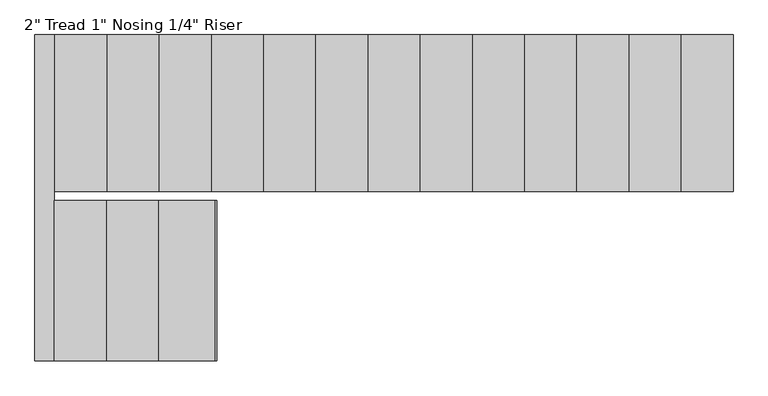
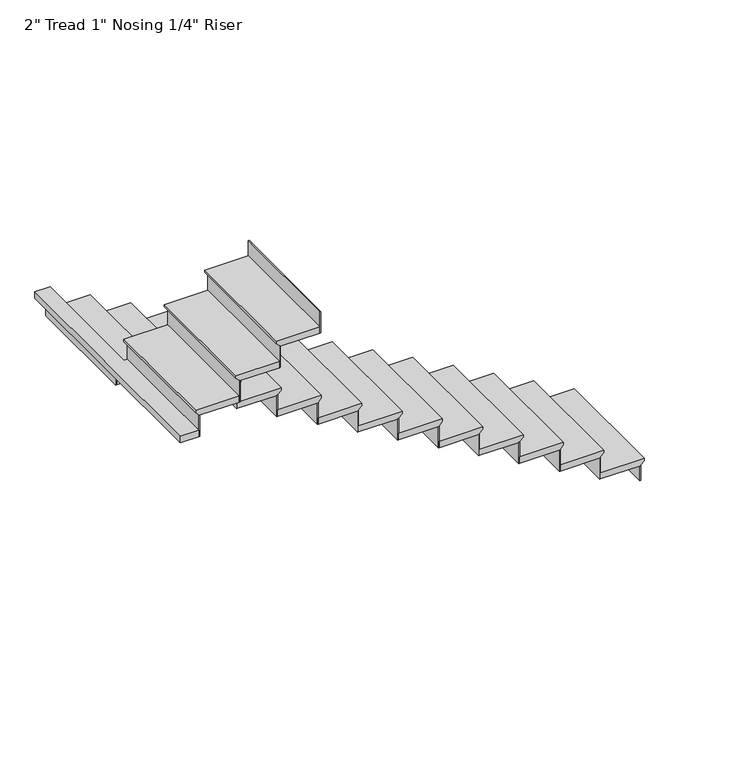
"""IFC4 building model written with IfcOpenShell, lengths in millimetres: stair flight geometry."""

from ifc_helpers import new_model, si_unit, origin, place, context, project, spatial, faceted_brep, source, transform, mapped, element, save


def stair_flight_91c59d30(model_context):
    return source(origin(), model_context, "Body", "Brep", [
        faceted_brep([(6794.5, 11386.0372886, 150.2833333), (6794.5, 11386.0372886, 169.3333333), (6794.5, 10471.6372886, 169.3333333), (6794.5, 10471.6372886, 150.2833333), (6769.1, 11386.0372886, 124.8833333), (6769.1, 10471.6372886, 124.8833333), (6464.3, 11386.0372886, 169.3333333), (6464.3, 10471.6372886, 169.3333333), (6769.1, 10471.6372886, 118.5333333), (6464.3, 10471.6372886, 118.5333333), (6464.3, 11386.0372886, 118.5333333), (6769.1, 11386.0372886, 118.5333333)], [[[0, 1, 2, 3]], [[4, 0, 3, 5]], [[2, 1, 6, 7]], [[8, 9, 10, 11]], [[2, 7, 9, 8, 5, 3]], [[8, 11, 4, 5]], [[6, 1, 0, 4, 11, 10]], [[7, 6, 10, 9]]]),
        faceted_brep([(6769.1, 11386.0372886, 118.5333333), (6769.1, 11386.0372886, 0.0), (6762.75, 11386.0372886, 0.0), (6762.75, 11386.0372886, 118.5333333), (6769.1, 10471.6372886, 118.5333333), (6762.75, 10471.6372886, 118.5333333), (6762.75, 10471.6372886, 0.0), (6769.1, 10471.6372886, 0.0)], [[[0, 1, 2, 3]], [[4, 5, 6, 7]], [[1, 0, 4, 7]], [[2, 1, 7, 6]], [[3, 2, 6, 5]], [[0, 3, 5, 4]]]),
        faceted_brep([(6464.3, 11386.0372886, 287.8666667), (6464.3, 11386.0372886, 118.5333333), (6457.95, 11386.0372886, 118.5333333), (6457.95, 11386.0372886, 287.8666667), (6464.3, 10471.6372886, 287.8666667), (6457.95, 10471.6372886, 287.8666667), (6457.95, 10471.6372886, 118.5333333), (6464.3, 10471.6372886, 118.5333333)], [[[0, 1, 2, 3]], [[4, 5, 6, 7]], [[1, 0, 4, 7]], [[2, 1, 7, 6]], [[3, 2, 6, 5]], [[0, 3, 5, 4]]]),
        faceted_brep([(6489.7, 10471.6372886, 338.6666667), (6489.7, 11386.0372886, 338.6666667), (6159.5, 11386.0372886, 338.6666667), (6159.5, 10471.6372886, 338.6666667), (6464.3, 10471.6372886, 287.8666667), (6159.5, 10471.6372886, 287.8666667), (6159.5, 11386.0372886, 287.8666667), (6464.3, 11386.0372886, 287.8666667), (6464.3, 10471.6372886, 294.2166667), (6489.7, 10471.6372886, 319.6166667), (6464.3, 11386.0372886, 294.2166667), (6489.7, 11386.0372886, 319.6166667)], [[[0, 1, 2, 3]], [[4, 5, 6, 7]], [[0, 3, 5, 4, 8, 9]], [[4, 7, 10, 8]], [[2, 1, 11, 10, 7, 6]], [[3, 2, 6, 5]], [[11, 1, 0, 9]], [[10, 11, 9, 8]]]),
        faceted_brep([(6159.5, 11386.0372886, 457.2), (6159.5, 11386.0372886, 287.8666667), (6153.15, 11386.0372886, 287.8666667), (6153.15, 11386.0372886, 457.2), (6159.5, 10471.6372886, 457.2), (6153.15, 10471.6372886, 457.2), (6153.15, 10471.6372886, 287.8666667), (6159.5, 10471.6372886, 287.8666667)], [[[0, 1, 2, 3]], [[4, 5, 6, 7]], [[1, 0, 4, 7]], [[2, 1, 7, 6]], [[3, 2, 6, 5]], [[0, 3, 5, 4]]]),
        faceted_brep([(6184.9, 10471.6372886, 508.0), (6184.9, 11386.0372886, 508.0), (5854.7, 11386.0372886, 508.0), (5854.7, 10471.6372886, 508.0), (6159.5, 10471.6372886, 457.2), (5854.7, 10471.6372886, 457.2), (5854.7, 11386.0372886, 457.2), (6159.5, 11386.0372886, 457.2), (6159.5, 10471.6372886, 463.55), (6184.9, 10471.6372886, 488.95), (6159.5, 11386.0372886, 463.55), (6184.9, 11386.0372886, 488.95)], [[[0, 1, 2, 3]], [[4, 5, 6, 7]], [[0, 3, 5, 4, 8, 9]], [[4, 7, 10, 8]], [[2, 1, 11, 10, 7, 6]], [[3, 2, 6, 5]], [[11, 1, 0, 9]], [[10, 11, 9, 8]]]),
        faceted_brep([(5854.7, 11386.0372886, 626.5333333), (5854.7, 11386.0372886, 457.2), (5848.35, 11386.0372886, 457.2), (5848.35, 11386.0372886, 626.5333333), (5854.7, 10471.6372886, 626.5333333), (5848.35, 10471.6372886, 626.5333333), (5848.35, 10471.6372886, 457.2), (5854.7, 10471.6372886, 457.2)], [[[0, 1, 2, 3]], [[4, 5, 6, 7]], [[1, 0, 4, 7]], [[2, 1, 7, 6]], [[3, 2, 6, 5]], [[0, 3, 5, 4]]]),
        faceted_brep([(5880.1, 10471.6372886, 677.3333333), (5880.1, 11386.0372886, 677.3333333), (5549.9, 11386.0372886, 677.3333333), (5549.9, 10471.6372886, 677.3333333), (5854.7, 10471.6372886, 626.5333333), (5549.9, 10471.6372886, 626.5333333), (5549.9, 11386.0372886, 626.5333333), (5854.7, 11386.0372886, 626.5333333), (5854.7, 10471.6372886, 632.8833333), (5880.1, 10471.6372886, 658.2833333), (5854.7, 11386.0372886, 632.8833333), (5880.1, 11386.0372886, 658.2833333)], [[[0, 1, 2, 3]], [[4, 5, 6, 7]], [[0, 3, 5, 4, 8, 9]], [[4, 7, 10, 8]], [[2, 1, 11, 10, 7, 6]], [[3, 2, 6, 5]], [[11, 1, 0, 9]], [[10, 11, 9, 8]]]),
        faceted_brep([(5549.9, 11386.0372886, 795.8666667), (5549.9, 11386.0372886, 626.5333333), (5543.55, 11386.0372886, 626.5333333), (5543.55, 11386.0372886, 795.8666667), (5549.9, 10471.6372886, 795.8666667), (5543.55, 10471.6372886, 795.8666667), (5543.55, 10471.6372886, 626.5333333), (5549.9, 10471.6372886, 626.5333333)], [[[0, 1, 2, 3]], [[4, 5, 6, 7]], [[1, 0, 4, 7]], [[2, 1, 7, 6]], [[3, 2, 6, 5]], [[0, 3, 5, 4]]]),
        faceted_brep([(5575.3, 10471.6372886, 846.6666667), (5575.3, 11386.0372886, 846.6666667), (5245.1, 11386.0372886, 846.6666667), (5245.1, 10471.6372886, 846.6666667), (5549.9, 10471.6372886, 795.8666667), (5245.1, 10471.6372886, 795.8666667), (5245.1, 11386.0372886, 795.8666667), (5549.9, 11386.0372886, 795.8666667), (5549.9, 10471.6372886, 802.2166667), (5575.3, 10471.6372886, 827.6166667), (5549.9, 11386.0372886, 802.2166667), (5575.3, 11386.0372886, 827.6166667)], [[[0, 1, 2, 3]], [[4, 5, 6, 7]], [[0, 3, 5, 4, 8, 9]], [[4, 7, 10, 8]], [[2, 1, 11, 10, 7, 6]], [[3, 2, 6, 5]], [[11, 1, 0, 9]], [[10, 11, 9, 8]]]),
        faceted_brep([(5245.1, 11386.0372886, 965.2), (5245.1, 11386.0372886, 795.8666667), (5238.75, 11386.0372886, 795.8666667), (5238.75, 11386.0372886, 965.2), (5245.1, 10471.6372886, 965.2), (5238.75, 10471.6372886, 965.2), (5238.75, 10471.6372886, 795.8666667), (5245.1, 10471.6372886, 795.8666667)], [[[0, 1, 2, 3]], [[4, 5, 6, 7]], [[1, 0, 4, 7]], [[2, 1, 7, 6]], [[3, 2, 6, 5]], [[0, 3, 5, 4]]]),
        faceted_brep([(5270.5, 10471.6372886, 1016.0), (5270.5, 11386.0372886, 1016.0), (4940.3, 11386.0372886, 1016.0), (4940.3, 10471.6372886, 1016.0), (5245.1, 10471.6372886, 965.2), (4940.3, 10471.6372886, 965.2), (4940.3, 11386.0372886, 965.2), (5245.1, 11386.0372886, 965.2), (5245.1, 10471.6372886, 971.55), (5270.5, 10471.6372886, 996.95), (5245.1, 11386.0372886, 971.55), (5270.5, 11386.0372886, 996.95)], [[[0, 1, 2, 3]], [[4, 5, 6, 7]], [[0, 3, 5, 4, 8, 9]], [[4, 7, 10, 8]], [[2, 1, 11, 10, 7, 6]], [[3, 2, 6, 5]], [[11, 1, 0, 9]], [[10, 11, 9, 8]]]),
        faceted_brep([(4940.3, 11386.0372886, 1134.5333333), (4940.3, 11386.0372886, 965.2), (4933.95, 11386.0372886, 965.2), (4933.95, 11386.0372886, 1134.5333333), (4940.3, 10471.6372886, 1134.5333333), (4933.95, 10471.6372886, 1134.5333333), (4933.95, 10471.6372886, 965.2), (4940.3, 10471.6372886, 965.2)], [[[0, 1, 2, 3]], [[4, 5, 6, 7]], [[1, 0, 4, 7]], [[2, 1, 7, 6]], [[3, 2, 6, 5]], [[0, 3, 5, 4]]]),
        faceted_brep([(4965.7, 10471.6372886, 1185.3333333), (4965.7, 11386.0372886, 1185.3333333), (4635.5, 11386.0372886, 1185.3333333), (4635.5, 10471.6372886, 1185.3333333), (4940.3, 10471.6372886, 1134.5333333), (4635.5, 10471.6372886, 1134.5333333), (4635.5, 11386.0372886, 1134.5333333), (4940.3, 11386.0372886, 1134.5333333), (4940.3, 10471.6372886, 1140.8833333), (4965.7, 10471.6372886, 1166.2833333), (4940.3, 11386.0372886, 1140.8833333), (4965.7, 11386.0372886, 1166.2833333)], [[[0, 1, 2, 3]], [[4, 5, 6, 7]], [[0, 3, 5, 4, 8, 9]], [[4, 7, 10, 8]], [[2, 1, 11, 10, 7, 6]], [[3, 2, 6, 5]], [[11, 1, 0, 9]], [[10, 11, 9, 8]]]),
        faceted_brep([(4635.5, 11386.0372886, 1303.8666667), (4635.5, 11386.0372886, 1134.5333333), (4629.15, 11386.0372886, 1134.5333333), (4629.15, 11386.0372886, 1303.8666667), (4635.5, 10471.6372886, 1303.8666667), (4629.15, 10471.6372886, 1303.8666667), (4629.15, 10471.6372886, 1134.5333333), (4635.5, 10471.6372886, 1134.5333333)], [[[0, 1, 2, 3]], [[4, 5, 6, 7]], [[1, 0, 4, 7]], [[2, 1, 7, 6]], [[3, 2, 6, 5]], [[0, 3, 5, 4]]]),
        faceted_brep([(4660.9, 10471.6372886, 1354.6666667), (4660.9, 11386.0372886, 1354.6666667), (4330.7, 11386.0372886, 1354.6666667), (4330.7, 10471.6372886, 1354.6666667), (4635.5, 10471.6372886, 1303.8666667), (4330.7, 10471.6372886, 1303.8666667), (4330.7, 11386.0372886, 1303.8666667), (4635.5, 11386.0372886, 1303.8666667), (4635.5, 10471.6372886, 1310.2166667), (4660.9, 10471.6372886, 1335.6166667), (4635.5, 11386.0372886, 1310.2166667), (4660.9, 11386.0372886, 1335.6166667)], [[[0, 1, 2, 3]], [[4, 5, 6, 7]], [[0, 3, 5, 4, 8, 9]], [[4, 7, 10, 8]], [[2, 1, 11, 10, 7, 6]], [[3, 2, 6, 5]], [[11, 1, 0, 9]], [[10, 11, 9, 8]]]),
        faceted_brep([(4330.7, 11386.0372886, 1473.2), (4330.7, 11386.0372886, 1303.8666667), (4324.35, 11386.0372886, 1303.8666667), (4324.35, 11386.0372886, 1473.2), (4330.7, 10471.6372886, 1473.2), (4324.35, 10471.6372886, 1473.2), (4324.35, 10471.6372886, 1303.8666667), (4330.7, 10471.6372886, 1303.8666667)], [[[0, 1, 2, 3]], [[4, 5, 6, 7]], [[1, 0, 4, 7]], [[2, 1, 7, 6]], [[3, 2, 6, 5]], [[0, 3, 5, 4]]]),
        faceted_brep([(4356.1, 10471.6372886, 1524.0), (4356.1, 11386.0372886, 1524.0), (4025.9, 11386.0372886, 1524.0), (4025.9, 10471.6372886, 1524.0), (4330.7, 10471.6372886, 1473.2), (4025.9, 10471.6372886, 1473.2), (4025.9, 11386.0372886, 1473.2), (4330.7, 11386.0372886, 1473.2), (4330.7, 10471.6372886, 1479.55), (4356.1, 10471.6372886, 1504.95), (4330.7, 11386.0372886, 1479.55), (4356.1, 11386.0372886, 1504.95)], [[[0, 1, 2, 3]], [[4, 5, 6, 7]], [[0, 3, 5, 4, 8, 9]], [[4, 7, 10, 8]], [[2, 1, 11, 10, 7, 6]], [[3, 2, 6, 5]], [[11, 1, 0, 9]], [[10, 11, 9, 8]]]),
        faceted_brep([(4025.9, 11386.0372886, 1642.5333333), (4025.9, 11386.0372886, 1473.2), (4019.55, 11386.0372886, 1473.2), (4019.55, 11386.0372886, 1642.5333333), (4025.9, 10471.6372886, 1642.5333333), (4019.55, 10471.6372886, 1642.5333333), (4019.55, 10471.6372886, 1473.2), (4025.9, 10471.6372886, 1473.2)], [[[0, 1, 2, 3]], [[4, 5, 6, 7]], [[1, 0, 4, 7]], [[2, 1, 7, 6]], [[3, 2, 6, 5]], [[0, 3, 5, 4]]]),
        faceted_brep([(4051.3, 10471.6372886, 1693.3333333), (4051.3, 11386.0372886, 1693.3333333), (3721.1, 11386.0372886, 1693.3333333), (3721.1, 10471.6372886, 1693.3333333), (4025.9, 10471.6372886, 1642.5333333), (3721.1, 10471.6372886, 1642.5333333), (3721.1, 11386.0372886, 1642.5333333), (4025.9, 11386.0372886, 1642.5333333), (4025.9, 10471.6372886, 1648.8833333), (4051.3, 10471.6372886, 1674.2833333), (4025.9, 11386.0372886, 1648.8833333), (4051.3, 11386.0372886, 1674.2833333)], [[[0, 1, 2, 3]], [[4, 5, 6, 7]], [[0, 3, 5, 4, 8, 9]], [[4, 7, 10, 8]], [[2, 1, 11, 10, 7, 6]], [[3, 2, 6, 5]], [[11, 1, 0, 9]], [[10, 11, 9, 8]]]),
        faceted_brep([(3721.1, 11386.0372886, 1811.8666667), (3721.1, 11386.0372886, 1642.5333333), (3714.75, 11386.0372886, 1642.5333333), (3714.75, 11386.0372886, 1811.8666667), (3721.1, 10471.6372886, 1811.8666667), (3714.75, 10471.6372886, 1811.8666667), (3714.75, 10471.6372886, 1642.5333333), (3721.1, 10471.6372886, 1642.5333333)], [[[0, 1, 2, 3]], [[4, 5, 6, 7]], [[1, 0, 4, 7]], [[2, 1, 7, 6]], [[3, 2, 6, 5]], [[0, 3, 5, 4]]]),
        faceted_brep([(3746.5, 10471.6372886, 1862.6666667), (3746.5, 11386.0372886, 1862.6666667), (3416.3, 11386.0372886, 1862.6666667), (3416.3, 10471.6372886, 1862.6666667), (3721.1, 10471.6372886, 1811.8666667), (3416.3, 10471.6372886, 1811.8666667), (3416.3, 11386.0372886, 1811.8666667), (3721.1, 11386.0372886, 1811.8666667), (3721.1, 10471.6372886, 1818.2166667), (3746.5, 10471.6372886, 1843.6166667), (3721.1, 11386.0372886, 1818.2166667), (3746.5, 11386.0372886, 1843.6166667)], [[[0, 1, 2, 3]], [[4, 5, 6, 7]], [[0, 3, 5, 4, 8, 9]], [[4, 7, 10, 8]], [[2, 1, 11, 10, 7, 6]], [[3, 2, 6, 5]], [[11, 1, 0, 9]], [[10, 11, 9, 8]]]),
        faceted_brep([(3416.3, 11386.0372886, 1981.2), (3416.3, 11386.0372886, 1811.8666667), (3409.95, 11386.0372886, 1811.8666667), (3409.95, 11386.0372886, 1981.2), (3416.3, 10471.6372886, 1981.2), (3409.95, 10471.6372886, 1981.2), (3409.95, 10471.6372886, 1811.8666667), (3416.3, 10471.6372886, 1811.8666667)], [[[0, 1, 2, 3]], [[4, 5, 6, 7]], [[1, 0, 4, 7]], [[2, 1, 7, 6]], [[3, 2, 6, 5]], [[0, 3, 5, 4]]]),
        faceted_brep([(3441.7, 10471.6372886, 2032.0), (3441.7, 11386.0372886, 2032.0), (3111.5, 11386.0372886, 2032.0), (3111.5, 10471.6372886, 2032.0), (3416.3, 10471.6372886, 1981.2), (3111.5, 10471.6372886, 1981.2), (3111.5, 11386.0372886, 1981.2), (3416.3, 11386.0372886, 1981.2), (3416.3, 10471.6372886, 1987.55), (3441.7, 10471.6372886, 2012.95), (3416.3, 11386.0372886, 1987.55), (3441.7, 11386.0372886, 2012.95)], [[[0, 1, 2, 3]], [[4, 5, 6, 7]], [[0, 3, 5, 4, 8, 9]], [[4, 7, 10, 8]], [[2, 1, 11, 10, 7, 6]], [[3, 2, 6, 5]], [[11, 1, 0, 9]], [[10, 11, 9, 8]]]),
        faceted_brep([(3111.5, 11386.0372886, 2150.5333333), (3111.5, 11386.0372886, 1981.2), (3105.15, 11386.0372886, 1981.2), (3105.15, 11386.0372886, 2150.5333333), (3111.5, 10471.6372886, 2150.5333333), (3105.15, 10471.6372886, 2150.5333333), (3105.15, 10471.6372886, 1981.2), (3111.5, 10471.6372886, 1981.2)], [[[0, 1, 2, 3]], [[4, 5, 6, 7]], [[1, 0, 4, 7]], [[2, 1, 7, 6]], [[3, 2, 6, 5]], [[0, 3, 5, 4]]]),
        faceted_brep([(3136.9, 10471.6372886, 2201.3333333), (3136.9, 11386.0372886, 2201.3333333), (2806.7, 11386.0372886, 2201.3333333), (2806.7, 10471.6372886, 2201.3333333), (3111.5, 10471.6372886, 2150.5333333), (2806.7, 10471.6372886, 2150.5333333), (2806.7, 11386.0372886, 2150.5333333), (3111.5, 11386.0372886, 2150.5333333), (3111.5, 10471.6372886, 2156.8833333), (3136.9, 10471.6372886, 2182.2833333), (3111.5, 11386.0372886, 2156.8833333), (3136.9, 11386.0372886, 2182.2833333)], [[[0, 1, 2, 3]], [[4, 5, 6, 7]], [[0, 3, 5, 4, 8, 9]], [[4, 7, 10, 8]], [[2, 1, 11, 10, 7, 6]], [[3, 2, 6, 5]], [[11, 1, 0, 9]], [[10, 11, 9, 8]]]),
        faceted_brep([(2806.7, 11386.0372886, 2319.8666667), (2806.7, 11386.0372886, 2150.5333333), (2800.35, 11386.0372886, 2150.5333333), (2800.35, 11386.0372886, 2319.8666667), (2806.7, 10471.6372886, 2319.8666667), (2800.35, 10471.6372886, 2319.8666667), (2800.35, 10471.6372886, 2150.5333333), (2806.7, 10471.6372886, 2150.5333333)], [[[0, 1, 2, 3]], [[4, 5, 6, 7]], [[1, 0, 4, 7]], [[2, 1, 7, 6]], [[3, 2, 6, 5]], [[0, 3, 5, 4]]]),
        faceted_brep([(2857.5, 10418.2972886, 2370.6666667), (2832.1, 10418.2972886, 2370.6666667), (2832.1, 11386.0372886, 2370.6666667), (2717.8, 11386.0372886, 2370.6666667), (2717.8, 9481.0372886, 2370.6666667), (2857.5, 9481.0372886, 2370.6666667), (2832.1, 10418.2972886, 2319.8666667), (2857.5, 10418.2972886, 2319.8666667), (2857.5, 9481.0372886, 2319.8666667), (2717.8, 9481.0372886, 2319.8666667), (2717.8, 11386.0372886, 2319.8666667), (2806.7, 11386.0372886, 2319.8666667), (2806.7, 10471.6372886, 2319.8666667), (2832.1, 10471.6372886, 2319.8666667), (2832.1, 10471.6372886, 2351.6166667), (2832.1, 11386.0372886, 2351.6166667), (2806.7, 10471.6372886, 2326.2166667), (2806.7, 11386.0372886, 2326.2166667)], [[[0, 1, 2, 3, 4, 5]], [[6, 7, 8, 9, 10, 11, 12, 13]], [[1, 0, 7, 6]], [[2, 1, 6, 13, 14, 15]], [[13, 12, 16, 14]], [[12, 11, 17, 16]], [[3, 2, 15, 17, 11, 10]], [[4, 3, 10, 9]], [[5, 4, 9, 8]], [[0, 5, 8, 7]], [[17, 15, 14, 16]]]),
        faceted_brep([(2857.5, 9481.0372886, 2489.2), (2857.5, 9481.0372886, 2319.8666667), (2863.85, 9481.0372886, 2319.8666667), (2863.85, 9481.0372886, 2489.2), (2857.5, 10418.2972886, 2489.2), (2863.85, 10418.2972886, 2489.2), (2863.85, 10418.2972886, 2319.8666667), (2857.5, 10418.2972886, 2319.8666667)], [[[0, 1, 2, 3]], [[4, 5, 6, 7]], [[1, 0, 4, 7]], [[2, 1, 7, 6]], [[3, 2, 6, 5]], [[0, 3, 5, 4]]]),
        faceted_brep([(2832.1, 10418.2972886, 2540.0), (2832.1, 9481.0372886, 2540.0), (3162.3, 9481.0372886, 2540.0), (3162.3, 10418.2972886, 2540.0), (2857.5, 10418.2972886, 2489.2), (3162.3, 10418.2972886, 2489.2), (3162.3, 9481.0372886, 2489.2), (2857.5, 9481.0372886, 2489.2), (2857.5, 10418.2972886, 2495.55), (2832.1, 10418.2972886, 2520.95), (2857.5, 9481.0372886, 2495.55), (2832.1, 9481.0372886, 2520.95)], [[[0, 1, 2, 3]], [[4, 5, 6, 7]], [[0, 3, 5, 4, 8, 9]], [[4, 7, 10, 8]], [[2, 1, 11, 10, 7, 6]], [[3, 2, 6, 5]], [[11, 1, 0, 9]], [[10, 11, 9, 8]]]),
        faceted_brep([(3162.3, 9481.0372886, 2658.5333333), (3162.3, 9481.0372886, 2489.2), (3168.65, 9481.0372886, 2489.2), (3168.65, 9481.0372886, 2658.5333333), (3162.3, 10418.2972886, 2658.5333333), (3168.65, 10418.2972886, 2658.5333333), (3168.65, 10418.2972886, 2489.2), (3162.3, 10418.2972886, 2489.2)], [[[0, 1, 2, 3]], [[4, 5, 6, 7]], [[1, 0, 4, 7]], [[2, 1, 7, 6]], [[3, 2, 6, 5]], [[0, 3, 5, 4]]]),
        faceted_brep([(3136.9, 10418.2972886, 2709.3333333), (3136.9, 9481.0372886, 2709.3333333), (3467.1, 9481.0372886, 2709.3333333), (3467.1, 10418.2972886, 2709.3333333), (3162.3, 10418.2972886, 2658.5333333), (3467.1, 10418.2972886, 2658.5333333), (3467.1, 9481.0372886, 2658.5333333), (3162.3, 9481.0372886, 2658.5333333), (3162.3, 10418.2972886, 2664.8833333), (3136.9, 10418.2972886, 2690.2833333), (3162.3, 9481.0372886, 2664.8833333), (3136.9, 9481.0372886, 2690.2833333)], [[[0, 1, 2, 3]], [[4, 5, 6, 7]], [[0, 3, 5, 4, 8, 9]], [[4, 7, 10, 8]], [[2, 1, 11, 10, 7, 6]], [[3, 2, 6, 5]], [[11, 1, 0, 9]], [[10, 11, 9, 8]]]),
        faceted_brep([(3467.1, 9481.0372886, 2827.8666667), (3467.1, 9481.0372886, 2658.5333333), (3473.45, 9481.0372886, 2658.5333333), (3473.45, 9481.0372886, 2827.8666667), (3467.1, 10418.2972886, 2827.8666667), (3473.45, 10418.2972886, 2827.8666667), (3473.45, 10418.2972886, 2658.5333333), (3467.1, 10418.2972886, 2658.5333333)], [[[0, 1, 2, 3]], [[4, 5, 6, 7]], [[1, 0, 4, 7]], [[2, 1, 7, 6]], [[3, 2, 6, 5]], [[0, 3, 5, 4]]]),
        faceted_brep([(3771.9019847, 9481.0372886, 2997.2), (3771.9019847, 9481.0372886, 2827.8666667), (3778.2519847, 9481.0372886, 2827.8666667), (3778.2519847, 9481.0372886, 2997.2), (3771.9019847, 10418.2972886, 2997.2), (3778.2519847, 10418.2972886, 2997.2), (3778.2519847, 10418.2972886, 2827.8666667), (3771.9019847, 10418.2972886, 2827.8666667)], [[[0, 1, 2, 3]], [[4, 5, 6, 7]], [[1, 0, 4, 7]], [[2, 1, 7, 6]], [[3, 2, 6, 5]], [[0, 3, 5, 4]]]),
        faceted_brep([(3441.7, 10418.2972886, 2878.6666667), (3441.7, 9481.0372886, 2878.6666667), (3771.9019847, 9481.0372886, 2878.6666667), (3771.9019847, 10418.2972886, 2878.6666667), (3467.1, 10418.2972886, 2827.8666667), (3771.9019847, 10418.2972886, 2827.8666667), (3771.9019847, 9481.0372886, 2827.8666667), (3467.1, 9481.0372886, 2827.8666667), (3467.1, 10418.2972886, 2834.2166667), (3441.7, 10418.2972886, 2859.6166667), (3467.1, 9481.0372886, 2834.2166667), (3441.7, 9481.0372886, 2859.6166667)], [[[0, 1, 2, 3]], [[4, 5, 6, 7]], [[0, 3, 5, 4, 8, 9]], [[4, 7, 10, 8]], [[2, 1, 11, 10, 7, 6]], [[3, 2, 6, 5]], [[11, 1, 0, 9]], [[10, 11, 9, 8]]]),
    ])


if __name__ == "__main__":
    model = new_model("IFC4")
    model_context = context("Model", 3, world=origin())
    ifc_project = project(units=[si_unit("LENGTHUNIT", "METRE", prefix="MILLI")], contexts=[model_context])
    site = spatial("IfcSite", under=ifc_project)
    building = spatial("IfcBuilding", under=site)
    placement = place(None, origin())
    stair_flight_shape = stair_flight_91c59d30(model_context)
    element("IfcStairFlight", 1, ObjectType="2\" Tread 1\" Nosing 1/4\" Riser", at=placement, inside=building, context=model_context, shape_type="MappedRepresentation", body=[
        mapped(stair_flight_shape, transform((0.0, 0.0, 0.0), x_axis=(1.0, 0.0, 0.0), y_axis=(0.0, 1.0, 0.0), z_axis=(0.0, 0.0, 1.0))),
    ])
    save(model, "model.ifc")
